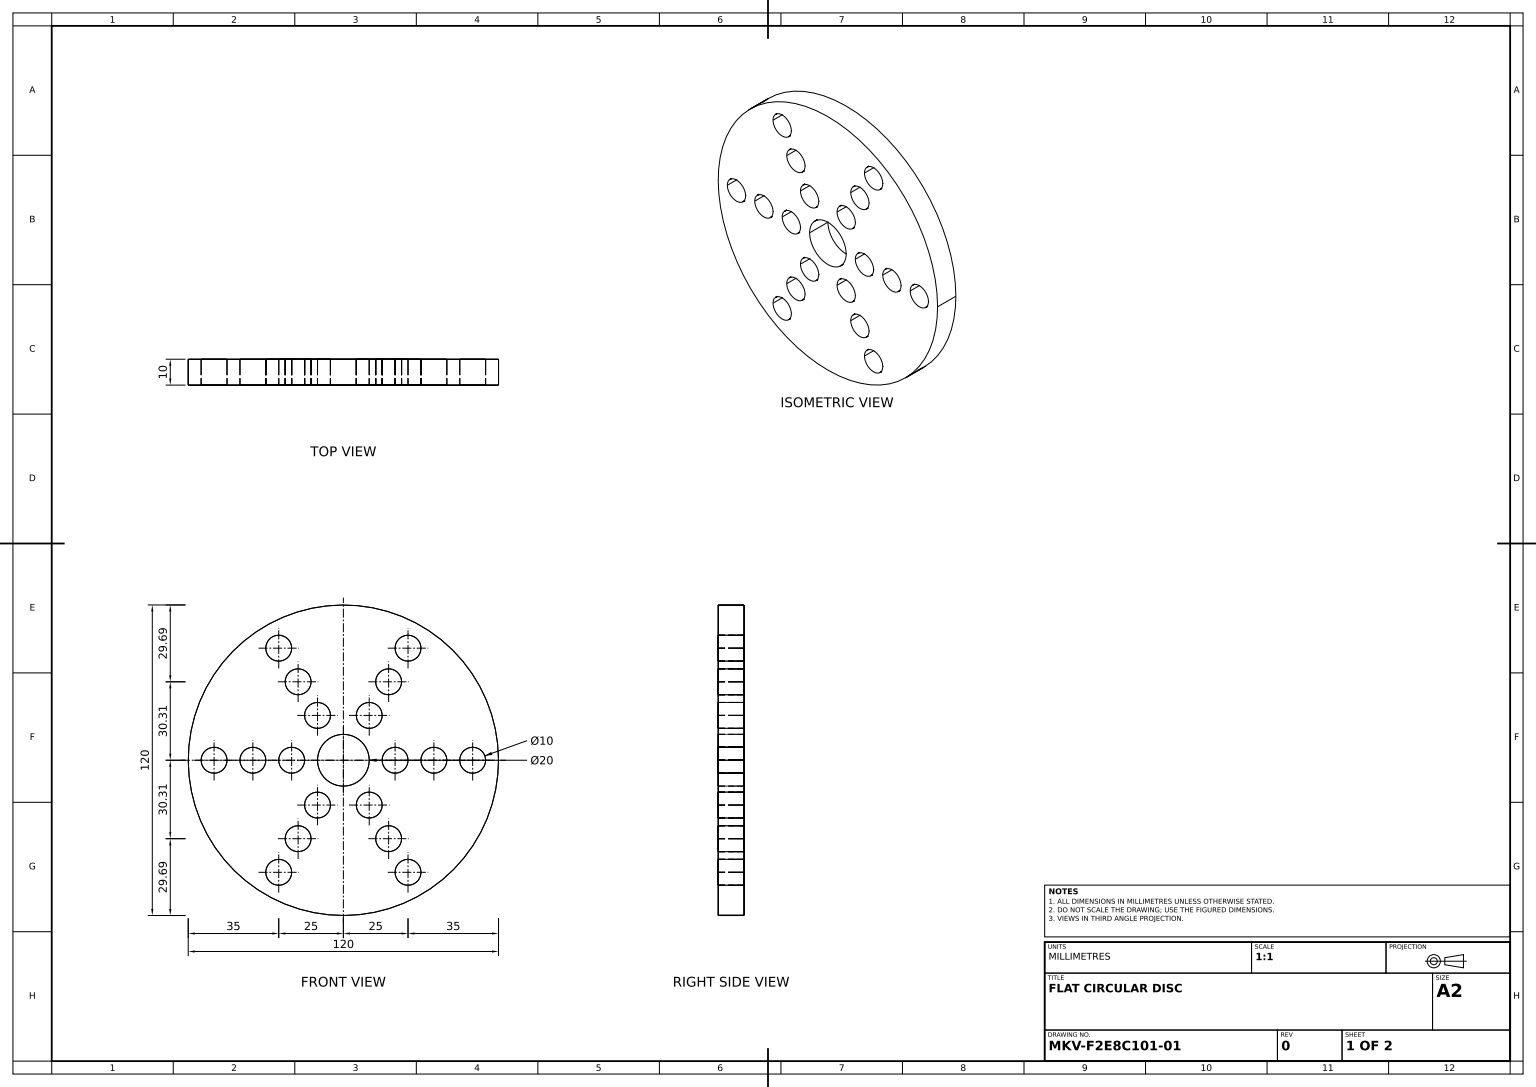
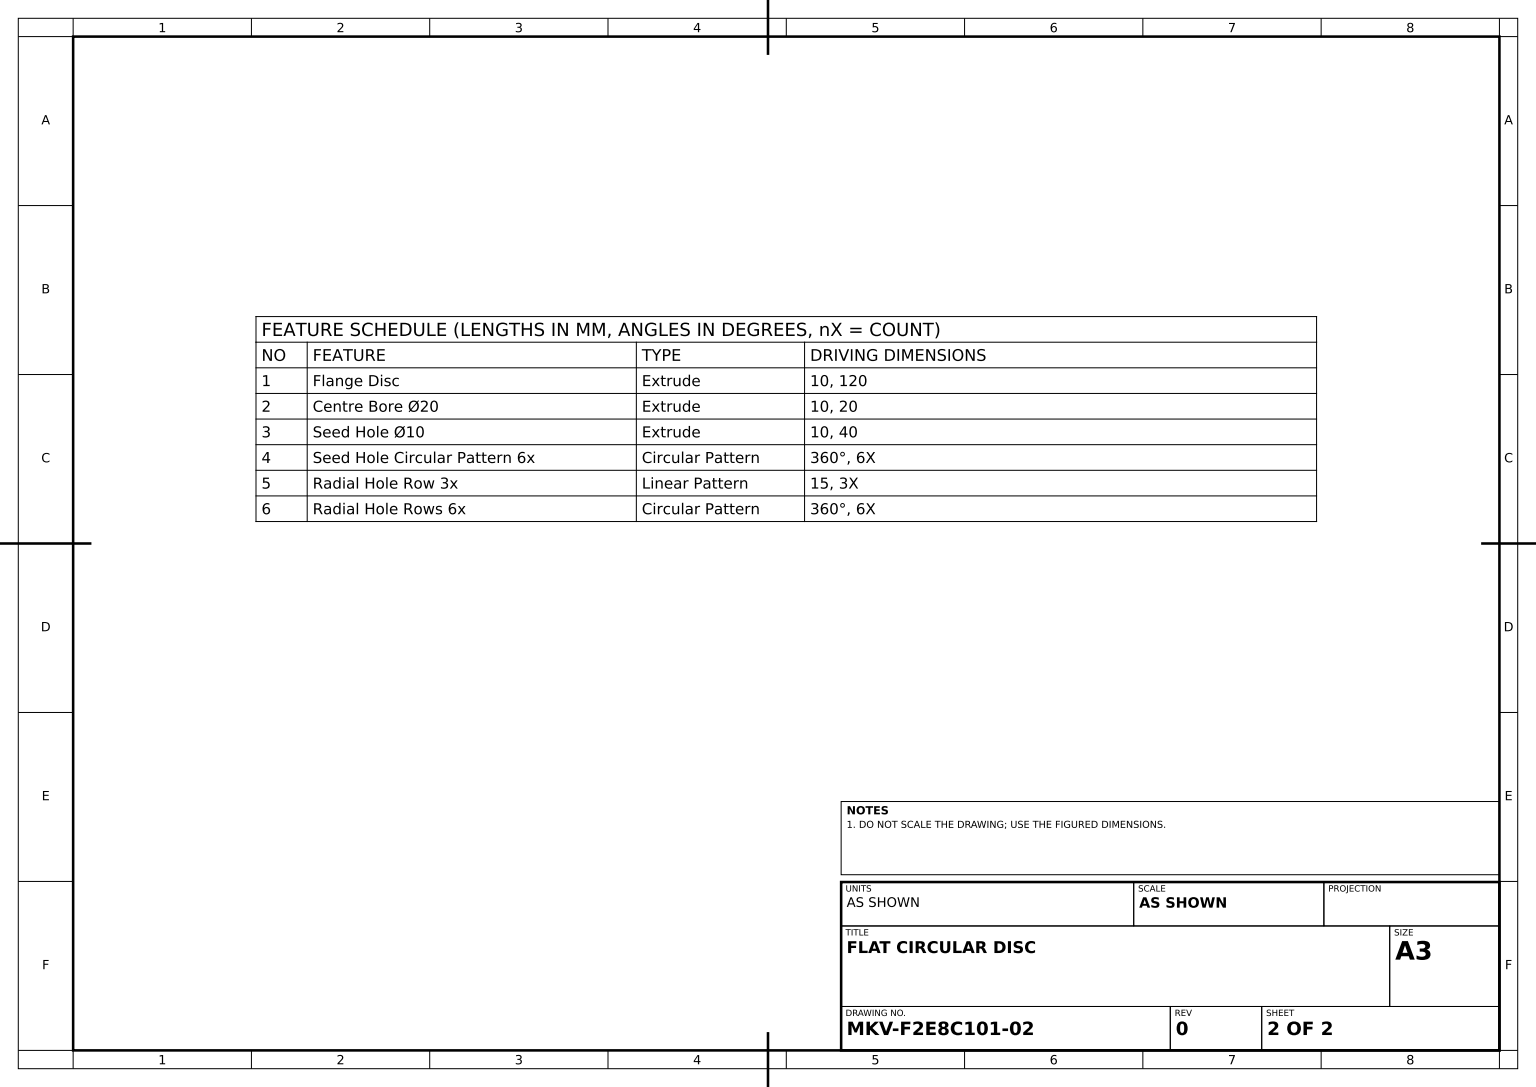
from build123d import *

# Parameters (mm, degrees)
FLANGE_OUTLINE_120_R                 = 60
FLANGE_DISC_DEPTH                    = 10
CENTRE_BORE_PROFILE_20_R             = 10
CENTRE_BORE_20_DEPTH                 = 10
SEED_HOLE_PROFILE_10_R               = 5
SEED_HOLE_10_DEPTH                   = 10
SEED_HOLE_CIRCULAR_PATTERN_6X_COUNT  = 6
RADIAL_HOLE_ROW_3X_COUNT             = 3
RADIAL_HOLE_ROW_3X_PITCH             = 15
RADIAL_HOLE_ROWS_6X_COPY_1_SKETCH_R  = 5
RADIAL_HOLE_ROWS_6X_COPY_1_DEPTH     = 10
RADIAL_HOLE_ROWS_6X_COPY_2_SKETCH_R  = 5
RADIAL_HOLE_ROWS_6X_COPY_2_DEPTH     = 10
RADIAL_HOLE_ROWS_6X_COPY_3_SKETCH_R  = 5
RADIAL_HOLE_ROWS_6X_COPY_3_DEPTH     = 10
RADIAL_HOLE_ROWS_6X_COPY_4_SKETCH_R  = 5
RADIAL_HOLE_ROWS_6X_COPY_4_DEPTH     = 10
RADIAL_HOLE_ROWS_6X_COPY_5_SKETCH_R  = 5
RADIAL_HOLE_ROWS_6X_COPY_5_DEPTH     = 10
RADIAL_HOLE_ROWS_6X_COPY_6_SKETCH_R  = 5
RADIAL_HOLE_ROWS_6X_COPY_6_DEPTH     = 10
RADIAL_HOLE_ROWS_6X_COPY_7_SKETCH_R  = 5
RADIAL_HOLE_ROWS_6X_COPY_7_DEPTH     = 10
RADIAL_HOLE_ROWS_6X_COPY_8_SKETCH_R  = 5
RADIAL_HOLE_ROWS_6X_COPY_8_DEPTH     = 10
RADIAL_HOLE_ROWS_6X_COPY_9_SKETCH_R  = 5
RADIAL_HOLE_ROWS_6X_COPY_9_DEPTH     = 10
RADIAL_HOLE_ROWS_6X_COPY_10_SKETCH_R = 5
RADIAL_HOLE_ROWS_6X_COPY_10_DEPTH    = 10
RADIAL_HOLE_ROWS_6X_COPY_11_SKETCH_R = 5
RADIAL_HOLE_ROWS_6X_COPY_11_DEPTH    = 10
RADIAL_HOLE_ROWS_6X_COPY_12_SKETCH_R = 5
RADIAL_HOLE_ROWS_6X_COPY_12_DEPTH    = 10
RADIAL_HOLE_ROWS_6X_COPY_13_SKETCH_R = 5
RADIAL_HOLE_ROWS_6X_COPY_13_DEPTH    = 10
RADIAL_HOLE_ROWS_6X_COPY_14_SKETCH_R = 5
RADIAL_HOLE_ROWS_6X_COPY_14_DEPTH    = 10
RADIAL_HOLE_ROWS_6X_COPY_15_SKETCH_R = 5
RADIAL_HOLE_ROWS_6X_COPY_15_DEPTH    = 10


with BuildPart() as part:
    # Flange Outline Ø120 → Flange Disc (new body)
    with BuildSketch(Plane.XY):
        Circle(FLANGE_OUTLINE_120_R)
    extrude(amount=FLANGE_DISC_DEPTH)

    # Centre Bore Profile Ø20 → Centre Bore Ø20 (cut)
    with BuildSketch(Plane.XY.offset(10)):
        Circle(CENTRE_BORE_PROFILE_20_R)
    extrude(amount=-CENTRE_BORE_20_DEPTH, mode=Mode.SUBTRACT)

    # Seed Hole Profile Ø10 → Seed Hole Ø10 (cut)
    with BuildSketch(Plane.XY.offset(10)):
        with Locations((20, 0)):
            Circle(SEED_HOLE_PROFILE_10_R)
    seed_hole_10 = extrude(amount=-SEED_HOLE_10_DEPTH, mode=Mode.SUBTRACT)

    # Seed Hole Circular Pattern 6x: Seed Hole Ø10 ×6 about axis
    seed_hole_circular_pattern_6x_axis = Axis((0, 0, 0), (0, 0, 1))
    for i in range(1, SEED_HOLE_CIRCULAR_PATTERN_6X_COUNT):
        add(seed_hole_10.rotate(seed_hole_circular_pattern_6x_axis, i * 360 / SEED_HOLE_CIRCULAR_PATTERN_6X_COUNT), mode=Mode.SUBTRACT)

    # Radial Hole Row 3x: Seed Hole Ø10 ×3
    with Locations(*[(i * RADIAL_HOLE_ROW_3X_PITCH, 0, 0) for i in range(1, RADIAL_HOLE_ROW_3X_COUNT)]):
        add(seed_hole_10, mode=Mode.SUBTRACT)

    # Radial Hole Rows 6x copy 1 sketch → Radial Hole Rows 6x copy 1 (cut)
    with BuildSketch(Plane(origin=(7.5, 12.990381057, 10), x_dir=(0.5000000000000001, 0.8660254037844386, 0), z_dir=(0, 0, 1))):
        with Locations((20, 0)):
            Circle(RADIAL_HOLE_ROWS_6X_COPY_1_SKETCH_R)
    extrude(amount=-RADIAL_HOLE_ROWS_6X_COPY_1_DEPTH, mode=Mode.SUBTRACT)

    # Radial Hole Rows 6x copy 2 sketch → Radial Hole Rows 6x copy 2 (cut)
    with BuildSketch(Plane(origin=(-7.5, 12.990381057, 10), x_dir=(-0.4999999999999998, 0.8660254037844387, 0), z_dir=(0, 0, 1))):
        with Locations((20, 0)):
            Circle(RADIAL_HOLE_ROWS_6X_COPY_2_SKETCH_R)
    extrude(amount=-RADIAL_HOLE_ROWS_6X_COPY_2_DEPTH, mode=Mode.SUBTRACT)

    # Radial Hole Rows 6x copy 3 sketch → Radial Hole Rows 6x copy 3 (cut)
    with BuildSketch(Plane(origin=(-15, 0, 10), x_dir=(-1, 0, 0), z_dir=(0, 0, 1))):
        with Locations((20, 0)):
            Circle(RADIAL_HOLE_ROWS_6X_COPY_3_SKETCH_R)
    extrude(amount=-RADIAL_HOLE_ROWS_6X_COPY_3_DEPTH, mode=Mode.SUBTRACT)

    # Radial Hole Rows 6x copy 4 sketch → Radial Hole Rows 6x copy 4 (cut)
    with BuildSketch(Plane(origin=(-7.5, -12.990381057, 10), x_dir=(-0.5000000000000004, -0.8660254037844384, 0), z_dir=(0, 0, 1))):
        with Locations((20, 0)):
            Circle(RADIAL_HOLE_ROWS_6X_COPY_4_SKETCH_R)
    extrude(amount=-RADIAL_HOLE_ROWS_6X_COPY_4_DEPTH, mode=Mode.SUBTRACT)

    # Radial Hole Rows 6x copy 5 sketch → Radial Hole Rows 6x copy 5 (cut)
    with BuildSketch(Plane(origin=(7.5, -12.990381057, 10), x_dir=(0.5000000000000001, -0.8660254037844386, 0), z_dir=(0, 0, 1))):
        with Locations((20, 0)):
            Circle(RADIAL_HOLE_ROWS_6X_COPY_5_SKETCH_R)
    extrude(amount=-RADIAL_HOLE_ROWS_6X_COPY_5_DEPTH, mode=Mode.SUBTRACT)

    # Radial Hole Rows 6x copy 6 sketch → Radial Hole Rows 6x copy 6 (cut)
    with BuildSketch(Plane(origin=(15, 25.980762114, 10), x_dir=(0.5000000000000001, 0.8660254037844386, 0), z_dir=(0, 0, 1))):
        with Locations((20, 0)):
            Circle(RADIAL_HOLE_ROWS_6X_COPY_6_SKETCH_R)
    extrude(amount=-RADIAL_HOLE_ROWS_6X_COPY_6_DEPTH, mode=Mode.SUBTRACT)

    # Radial Hole Rows 6x copy 7 sketch → Radial Hole Rows 6x copy 7 (cut)
    with BuildSketch(Plane(origin=(-15, 25.980762114, 10), x_dir=(-0.4999999999999998, 0.8660254037844387, 0), z_dir=(0, 0, 1))):
        with Locations((20, 0)):
            Circle(RADIAL_HOLE_ROWS_6X_COPY_7_SKETCH_R)
    extrude(amount=-RADIAL_HOLE_ROWS_6X_COPY_7_DEPTH, mode=Mode.SUBTRACT)

    # Radial Hole Rows 6x copy 8 sketch → Radial Hole Rows 6x copy 8 (cut)
    with BuildSketch(Plane(origin=(-30, 0, 10), x_dir=(-1, 0, 0), z_dir=(0, 0, 1))):
        with Locations((20, 0)):
            Circle(RADIAL_HOLE_ROWS_6X_COPY_8_SKETCH_R)
    extrude(amount=-RADIAL_HOLE_ROWS_6X_COPY_8_DEPTH, mode=Mode.SUBTRACT)

    # Radial Hole Rows 6x copy 9 sketch → Radial Hole Rows 6x copy 9 (cut)
    with BuildSketch(Plane(origin=(-15, -25.980762114, 10), x_dir=(-0.5000000000000004, -0.8660254037844384, 0), z_dir=(0, 0, 1))):
        with Locations((20, 0)):
            Circle(RADIAL_HOLE_ROWS_6X_COPY_9_SKETCH_R)
    extrude(amount=-RADIAL_HOLE_ROWS_6X_COPY_9_DEPTH, mode=Mode.SUBTRACT)

    # Radial Hole Rows 6x copy 10 sketch → Radial Hole Rows 6x copy 10 (cut)
    with BuildSketch(Plane(origin=(15, -25.980762114, 10), x_dir=(0.5000000000000001, -0.8660254037844386, 0), z_dir=(0, 0, 1))):
        with Locations((20, 0)):
            Circle(RADIAL_HOLE_ROWS_6X_COPY_10_SKETCH_R)
    extrude(amount=-RADIAL_HOLE_ROWS_6X_COPY_10_DEPTH, mode=Mode.SUBTRACT)

    # Radial Hole Rows 6x copy 11 sketch → Radial Hole Rows 6x copy 11 (cut)
    with BuildSketch(Plane(origin=(0, 0, 10), x_dir=(0.5000000000000001, 0.8660254037844386, 0), z_dir=(0, 0, 1))):
        with Locations((20, 0)):
            Circle(RADIAL_HOLE_ROWS_6X_COPY_11_SKETCH_R)
    extrude(amount=-RADIAL_HOLE_ROWS_6X_COPY_11_DEPTH, mode=Mode.SUBTRACT)

    # Radial Hole Rows 6x copy 12 sketch → Radial Hole Rows 6x copy 12 (cut)
    with BuildSketch(Plane(origin=(0, 0, 10), x_dir=(-0.4999999999999998, 0.8660254037844387, 0), z_dir=(0, 0, 1))):
        with Locations((20, 0)):
            Circle(RADIAL_HOLE_ROWS_6X_COPY_12_SKETCH_R)
    extrude(amount=-RADIAL_HOLE_ROWS_6X_COPY_12_DEPTH, mode=Mode.SUBTRACT)

    # Radial Hole Rows 6x copy 13 sketch → Radial Hole Rows 6x copy 13 (cut)
    with BuildSketch(Plane(origin=(0, 0, 10), x_dir=(-1, 0, 0), z_dir=(0, 0, 1))):
        with Locations((20, 0)):
            Circle(RADIAL_HOLE_ROWS_6X_COPY_13_SKETCH_R)
    extrude(amount=-RADIAL_HOLE_ROWS_6X_COPY_13_DEPTH, mode=Mode.SUBTRACT)

    # Radial Hole Rows 6x copy 14 sketch → Radial Hole Rows 6x copy 14 (cut)
    with BuildSketch(Plane(origin=(0, 0, 10), x_dir=(-0.5000000000000004, -0.8660254037844384, 0), z_dir=(0, 0, 1))):
        with Locations((20, 0)):
            Circle(RADIAL_HOLE_ROWS_6X_COPY_14_SKETCH_R)
    extrude(amount=-RADIAL_HOLE_ROWS_6X_COPY_14_DEPTH, mode=Mode.SUBTRACT)

    # Radial Hole Rows 6x copy 15 sketch → Radial Hole Rows 6x copy 15 (cut)
    with BuildSketch(Plane(origin=(0, 0, 10), x_dir=(0.5000000000000001, -0.8660254037844386, 0), z_dir=(0, 0, 1))):
        with Locations((20, 0)):
            Circle(RADIAL_HOLE_ROWS_6X_COPY_15_SKETCH_R)
    extrude(amount=-RADIAL_HOLE_ROWS_6X_COPY_15_DEPTH, mode=Mode.SUBTRACT)


solid = part.part
